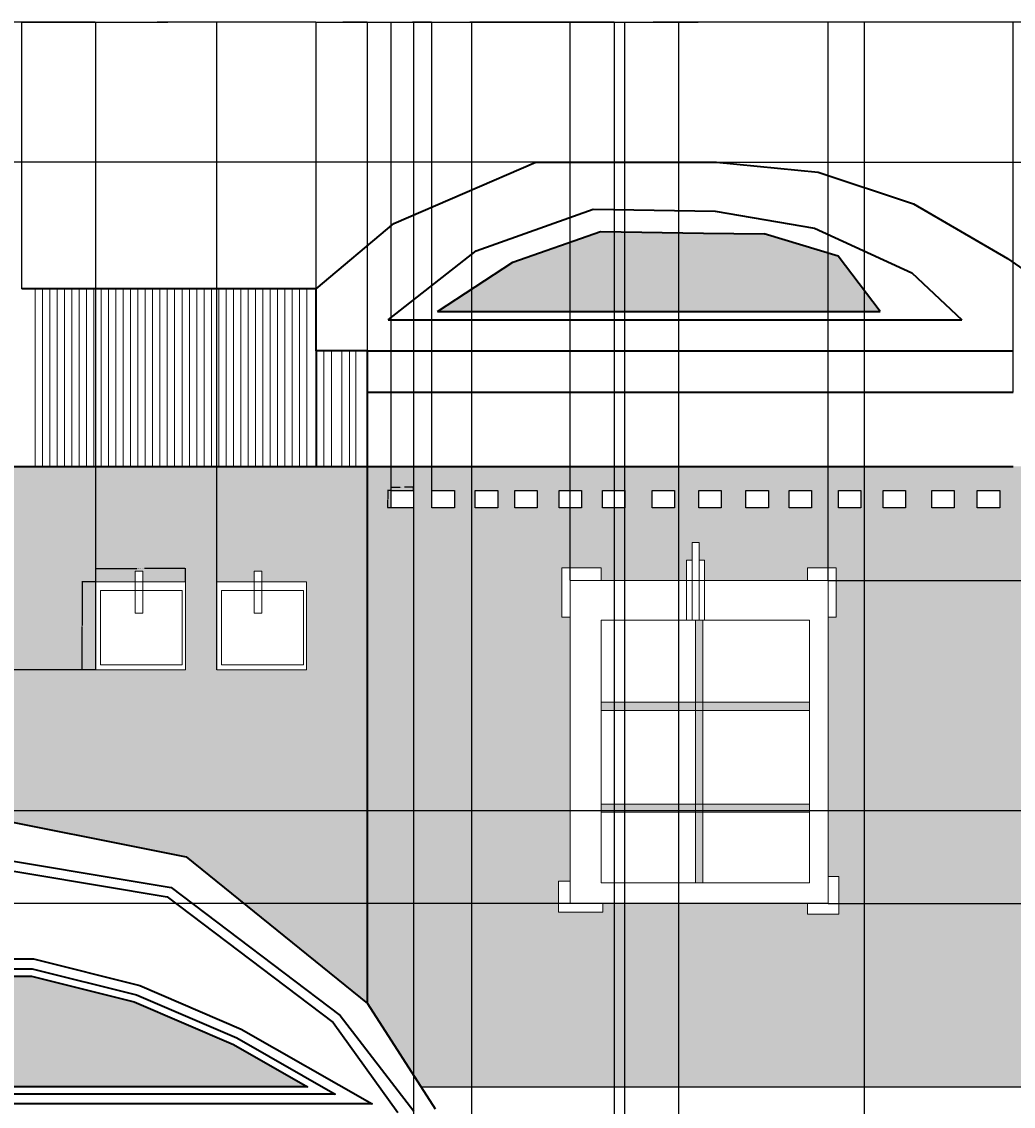
# Model space of a CAD drawing. Units: inches. Extents: x -46 to 1209, y 110 to 778.
# Tile 3 of 5: x 247 to 652, y 334 to 778. Entities that reach past the tile are written whole.
import ezdxf

# ---------------------------------------------------------------- set-up
doc = ezdxf.new("R2010")
doc.units = ezdxf.units.IN
doc.header["$MEASUREMENT"] = 0
for name, color, linetype, lineweight in [('A-ANNO-DIMS', 2, 'Continuous', 18), ('A-GLAZ', 4, 'Continuous', 20), ('A-GLAZ-PATT', 9, 'Continuous', 13), ('A-ROOF', 7, 'Continuous', 35), ('A-ROOF-PATT', 8, 'Continuous', 13), ('A-WALL', 7, 'Continuous', 35), ('A-WALL-PATT', 252, 'Continuous', 13), ('A-WALL-TRIM', 42, 'Continuous', 25)]:
    doc.layers.add(name, color=color, linetype=linetype, lineweight=lineweight)
doc.styles.get("Standard").update_dxf_attribs({"font": 'arial.ttf'})
doc.dimstyles.get("Standard").update_dxf_attribs({"dimtxt": 0.18, "dimasz": 0.18, "dimexe": 0.18, "dimexo": 0.0625, "dimgap": 0.09, "dimtad": 0, "dimtih": 1, "dimtoh": 1, "dimdec": 4, "dimzin": 0, "dimdsep": 46, "dimtxsty": 'Standard', "dimcen": 0.09, "dimadec": 0, "dimazin": 0, "dimtfac": 1, "dimtdec": 4, "dimtofl": 0, "dimtmove": 0, "dimatfit": 3, "dimfxl": 1, "dimtolj": 1, "dimtzin": 0, "dimarcsym": 0})

# ---------------------------------------------------------------- blocks, each defined once
blk = doc.blocks.new('WIN-SMALL-FRAME')
for points in [[(0, 35.97), (36.6, 35.97), (36.6, 0), (0, 0)], [(1.9, 32.4), (35.37, 32.4), (35.37, 2.05), (1.9, 2.05)]]:
    blk.add_lwpolyline(points, close=True)
blk = doc.blocks.new('DENTIL-FACADE')
blk.add_lwpolyline([(0, 7.16), (9.17, 7.16), (9.17, 0), (0, 0)], close=True)
blk = doc.blocks.new('*D12')
at = {"layer": 'A-ANNO-DIMS', "color": 0, "lineweight": -2, "transparency": 16777216}
for p, q in [((397.42, 586.03), (397.42, 587.53)), ((397.6, 587.35), (401.07, 587.35)), ((406.42, 587.35), (402.94, 587.35)), ((406.6, 586.03), (406.6, 587.53))]:
    blk.add_line(p, q, dxfattribs=at)
at = {"layer": 'A-ANNO-DIMS', "color": 0, "transparency": 16777216}
for points in [[(397.6, 587.38), (397.6, 587.32), (397.42, 587.35)], [(406.42, 587.38), (406.42, 587.32), (406.6, 587.35)]]:
    blk.add_solid(points, dxfattribs=at)
at = {"layer": 'Defpoints', "color": 0, "transparency": 16777216}
for p in [(397.42, 585.97), (406.6, 587.35), (406.6, 585.97)]:
    blk.add_point(p, dxfattribs=at)
at = {"layer": 'A-ANNO-DIMS', "color": 0, "transparency": 16777216, "insert": (402.01, 587.35), "char_height": 0.18, "attachment_point": 5}
blk.add_mtext('\\A1;DENTIL 9 TYP.', dxfattribs=at)
blk = doc.blocks.new('*D13')
at = {"layer": 'A-ANNO-DIMS', "color": 0, "lineweight": -2, "transparency": 16777216}
for p, q in [((397.36, 585.97), (395.87, 585.97)), ((396.05, 585.79), (396.05, 582.57)), ((396.05, 578.99), (396.05, 582.21)), ((397.36, 578.81), (395.87, 578.81))]:
    blk.add_line(p, q, dxfattribs=at)
at = {"layer": 'A-ANNO-DIMS', "color": 0, "transparency": 16777216}
for points in [[(396.02, 585.79), (396.08, 585.79), (396.05, 585.97)], [(396.02, 578.99), (396.08, 578.99), (396.05, 578.81)]]:
    blk.add_solid(points, dxfattribs=at)
at = {"layer": 'Defpoints', "color": 0, "transparency": 16777216}
for p in [(396.05, 585.97), (397.42, 585.97), (397.42, 578.81)]:
    blk.add_point(p, dxfattribs=at)
at = {"layer": 'A-ANNO-DIMS', "color": 0, "transparency": 16777216, "insert": (396.05, 582.39), "char_height": 0.18, "attachment_point": 5}
blk.add_mtext('\\A1;7 TYP.', dxfattribs=at)
blk = doc.blocks.new('*D20')
at = {"layer": 'A-ANNO-DIMS', "color": 0, "lineweight": -2, "transparency": 16777216}
for p, q in [((276.76, 548.66), (276.76, 554.27)), ((313.37, 548.66), (313.37, 554.27)), ((276.94, 554.09), (293.5, 554.09)), ((313.19, 554.09), (296.63, 554.09))]:
    blk.add_line(p, q, dxfattribs=at)
at = {"layer": 'A-ANNO-DIMS', "color": 0, "transparency": 16777216}
for points in [[(276.94, 554.12), (276.94, 554.06), (276.76, 554.09)], [(313.19, 554.12), (313.19, 554.06), (313.37, 554.09)]]:
    blk.add_solid(points, dxfattribs=at)
at = {"layer": 'Defpoints', "color": 0, "transparency": 16777216}
for p in [(313.37, 554.09), (276.76, 548.59), (313.37, 548.59)]:
    blk.add_point(p, dxfattribs=at)
at = {"layer": 'A-ANNO-DIMS', "color": 0, "transparency": 16777216, "insert": (295.07, 554.09), "char_height": 0.18, "attachment_point": 5}
blk.add_mtext('\\A1;SMALL WINDOW 37 TYP.', dxfattribs=at)
blk = doc.blocks.new('*D21')
at = {"layer": 'A-ANNO-DIMS', "color": 0, "lineweight": -2, "transparency": 16777216}
for p, q in [((276.7, 548.59), (271.09, 548.59)), ((271.27, 548.41), (271.27, 530.79)), ((271.27, 512.81), (271.27, 530.43)), ((276.7, 512.63), (271.09, 512.63))]:
    blk.add_line(p, q, dxfattribs=at)
at = {"layer": 'A-ANNO-DIMS', "color": 0, "transparency": 16777216}
for points in [[(271.24, 548.41), (271.3, 548.41), (271.27, 548.59)], [(271.24, 512.81), (271.3, 512.81), (271.27, 512.63)]]:
    blk.add_solid(points, dxfattribs=at)
at = {"layer": 'Defpoints', "color": 0, "transparency": 16777216}
for p in [(271.27, 548.59), (276.76, 548.59), (276.76, 512.63)]:
    blk.add_point(p, dxfattribs=at)
at = {"layer": 'A-ANNO-DIMS', "color": 0, "transparency": 16777216, "insert": (271.27, 530.61), "char_height": 0.18, "attachment_point": 5}
blk.add_mtext('\\A1;36 TYP.', dxfattribs=at)
blk = doc.blocks.new('*D29')
at = {"layer": 'A-ANNO-DIMS', "color": 0, "lineweight": -2, "transparency": 16777216}
for p, q in [((456.52, 720.07), (-45.5, 720.07)), ((-45.32, 719.89), (-45.32, 443.93)), ((-45.32, 167.62), (-45.32, 443.57)), ((15.16, 167.44), (-45.5, 167.44))]:
    blk.add_line(p, q, dxfattribs=at)
at = {"layer": 'A-ANNO-DIMS', "color": 0, "transparency": 16777216}
for points in [[(-45.35, 719.89), (-45.29, 719.89), (-45.32, 720.07)], [(-45.35, 167.62), (-45.29, 167.62), (-45.32, 167.44)]]:
    blk.add_solid(points, dxfattribs=at)
at = {"layer": 'Defpoints', "color": 0, "transparency": 16777216}
for p in [(-45.32, 720.07), (456.58, 720.07), (15.23, 167.44)]:
    blk.add_point(p, dxfattribs=at)
at = {"layer": 'A-ANNO-DIMS', "color": 0, "transparency": 16777216, "insert": (-45.32, 443.75), "char_height": 0.18, "attachment_point": 5}
blk.add_mtext('\\A1;552.6', dxfattribs=at)
blk = doc.blocks.new('*D46')
at = {"layer": 'A-ANNO-DIMS', "color": 0, "lineweight": -2, "transparency": 16777216}
for p, q in [((406.65, 322.05), (406.65, 777.55)), ((406.83, 777.37), (447.43, 777.37)), ((488.47, 777.37), (447.87, 777.37)), ((488.65, 273.58), (488.65, 777.55))]:
    blk.add_line(p, q, dxfattribs=at)
at = {"layer": 'A-ANNO-DIMS', "color": 0, "transparency": 16777216}
for points in [[(406.83, 777.4), (406.83, 777.34), (406.65, 777.37)], [(488.47, 777.4), (488.47, 777.34), (488.65, 777.37)]]:
    blk.add_solid(points, dxfattribs=at)
at = {"layer": 'Defpoints', "color": 0, "transparency": 16777216}
for p in [(488.65, 777.37), (406.65, 321.99), (488.65, 273.51)]:
    blk.add_point(p, dxfattribs=at)
at = {"layer": 'A-ANNO-DIMS', "color": 0, "transparency": 16777216, "insert": (447.65, 777.37), "char_height": 0.18, "attachment_point": 5}
blk.add_mtext('\\A1;82', dxfattribs=at)
blk = doc.blocks.new('*D50')
at = {"layer": 'A-ANNO-DIMS', "color": 0, "lineweight": -2, "transparency": 16777216}
for p, q in [((430.32, 322.05), (430.32, 777.55)), ((430.5, 777.37), (510.13, 777.37)), ((590.53, 777.37), (510.9, 777.37)), ((590.71, 322.05), (590.71, 777.55))]:
    blk.add_line(p, q, dxfattribs=at)
at = {"layer": 'A-ANNO-DIMS', "color": 0, "transparency": 16777216}
for points in [[(430.5, 777.4), (430.5, 777.34), (430.32, 777.37)], [(590.53, 777.4), (590.53, 777.34), (590.71, 777.37)]]:
    blk.add_solid(points, dxfattribs=at)
at = {"layer": 'Defpoints', "color": 0, "transparency": 16777216}
for p in [(590.71, 777.37), (430.32, 321.99), (590.71, 321.99)]:
    blk.add_point(p, dxfattribs=at)
at = {"layer": 'A-ANNO-DIMS', "color": 0, "transparency": 16777216, "insert": (510.52, 777.37), "char_height": 0.18, "attachment_point": 5}
blk.add_mtext('\\A1;160.4', dxfattribs=at)
blk = doc.blocks.new('*D51')
at = {"layer": 'A-ANNO-DIMS', "color": 0, "lineweight": -2, "transparency": 16777216}
for p, q in [((492.93, 261.94), (492.93, 777.55)), ((493.11, 777.37), (503.47, 777.37)), ((514.76, 777.37), (504.4, 777.37)), ((514.94, 261.94), (514.94, 777.55))]:
    blk.add_line(p, q, dxfattribs=at)
at = {"layer": 'A-ANNO-DIMS', "color": 0, "transparency": 16777216}
for points in [[(493.11, 777.4), (493.11, 777.34), (492.93, 777.37)], [(514.76, 777.4), (514.76, 777.34), (514.94, 777.37)]]:
    blk.add_solid(points, dxfattribs=at)
at = {"layer": 'Defpoints', "color": 0, "transparency": 16777216}
for p in [(514.94, 777.37), (492.93, 261.87), (514.94, 261.87)]:
    blk.add_point(p, dxfattribs=at)
at = {"layer": 'A-ANNO-DIMS', "color": 0, "transparency": 16777216, "insert": (503.94, 777.37), "char_height": 0.18, "attachment_point": 5}
blk.add_mtext('\\A1;22.003', dxfattribs=at)
blk = doc.blocks.new('*D59')
at = {"layer": 'A-ANNO-DIMS', "color": 0, "lineweight": -2, "transparency": 16777216}
for p, q in [((530.31, 720.07), (1209.28, 720.07)), ((1209.1, 719.89), (1209.1, 694.37)), ((1209.1, 668.48), (1209.1, 694)), ((1091.9, 668.3), (1209.28, 668.3))]:
    blk.add_line(p, q, dxfattribs=at)
at = {"layer": 'A-ANNO-DIMS', "color": 0, "transparency": 16777216}
for points in [[(1209.07, 719.89), (1209.13, 719.89), (1209.1, 720.07)], [(1209.07, 668.48), (1209.13, 668.48), (1209.1, 668.3)]]:
    blk.add_solid(points, dxfattribs=at)
at = {"layer": 'Defpoints', "color": 0, "transparency": 16777216}
for p in [(530.25, 720.07), (1209.1, 720.07), (1091.84, 668.3)]:
    blk.add_point(p, dxfattribs=at)
at = {"layer": 'A-ANNO-DIMS', "color": 0, "transparency": 16777216, "insert": (1209.1, 694.19), "char_height": 0.18, "attachment_point": 5}
blk.add_mtext('\\A1;51.77', dxfattribs=at)
blk = doc.blocks.new('*D61')
at = {"layer": 'A-ANNO-DIMS', "color": 0, "lineweight": -2, "transparency": 16777216}
for p, q in [((179.04, 595.79), (-45.5, 595.79)), ((-45.32, 595.61), (-45.32, 554.39)), ((-45.32, 512.81), (-45.32, 554.03)), ((276.7, 512.63), (-45.5, 512.63))]:
    blk.add_line(p, q, dxfattribs=at)
at = {"layer": 'A-ANNO-DIMS', "color": 0, "transparency": 16777216}
for points in [[(-45.35, 595.61), (-45.29, 595.61), (-45.32, 595.79)], [(-45.35, 512.81), (-45.29, 512.81), (-45.32, 512.63)]]:
    blk.add_solid(points, dxfattribs=at)
at = {"layer": 'Defpoints', "color": 0, "transparency": 16777216}
for p in [(179.1, 595.79), (-45.32, 512.63), (276.76, 512.63)]:
    blk.add_point(p, dxfattribs=at)
at = {"layer": 'A-ANNO-DIMS', "color": 0, "transparency": 16777216, "insert": (-45.32, 554.21), "char_height": 0.18, "attachment_point": 5}
blk.add_mtext('\\A1;83.16', dxfattribs=at)
blk = doc.blocks.new('*D62')
at = {"layer": 'A-ANNO-DIMS', "color": 0, "lineweight": -2, "transparency": 16777216}
for p, q in [((179.1, 595.85), (179.1, 777.55)), ((179.28, 777.37), (227.54, 777.37)), ((276.58, 777.37), (228.33, 777.37)), ((276.76, 512.69), (276.76, 777.55))]:
    blk.add_line(p, q, dxfattribs=at)
at = {"layer": 'A-ANNO-DIMS', "color": 0, "transparency": 16777216}
for points in [[(179.28, 777.4), (179.28, 777.34), (179.1, 777.37)], [(276.58, 777.4), (276.58, 777.34), (276.76, 777.37)]]:
    blk.add_solid(points, dxfattribs=at)
at = {"layer": 'Defpoints', "color": 0, "transparency": 16777216}
for p in [(276.76, 777.37), (179.1, 595.79), (276.76, 512.63)]:
    blk.add_point(p, dxfattribs=at)
at = {"layer": 'A-ANNO-DIMS', "color": 0, "transparency": 16777216, "insert": (227.93, 777.37), "char_height": 0.18, "attachment_point": 5}
blk.add_mtext('\\A1;97.66', dxfattribs=at)
blk = doc.blocks.new('*D63')
at = {"layer": 'A-ANNO-DIMS', "color": 0, "lineweight": -2, "transparency": 16777216}
for p, q in [((276.76, 512.69), (276.76, 777.55)), ((276.94, 777.37), (301.19, 777.37)), ((326.09, 777.37), (301.84, 777.37)), ((326.27, 512.69), (326.27, 777.55))]:
    blk.add_line(p, q, dxfattribs=at)
at = {"layer": 'A-ANNO-DIMS', "color": 0, "transparency": 16777216}
for points in [[(276.94, 777.4), (276.94, 777.34), (276.76, 777.37)], [(326.09, 777.4), (326.09, 777.34), (326.27, 777.37)]]:
    blk.add_solid(points, dxfattribs=at)
at = {"layer": 'Defpoints', "color": 0, "transparency": 16777216}
for p in [(326.27, 777.37), (276.76, 512.63), (326.27, 512.63)]:
    blk.add_point(p, dxfattribs=at)
at = {"layer": 'A-ANNO-DIMS', "color": 0, "transparency": 16777216, "insert": (301.52, 777.37), "char_height": 0.18, "attachment_point": 5}
blk.add_mtext('\\A1;49.5', dxfattribs=at)
blk = doc.blocks.new('*D64')
at = {"layer": 'A-ANNO-DIMS', "color": 0, "lineweight": -2, "transparency": 16777216}
for p, q in [((387.83, 595.85), (387.83, 777.55)), ((388.01, 777.37), (428.78, 777.37)), ((470.33, 777.37), (429.56, 777.37)), ((470.51, 549.26), (470.51, 777.55))]:
    blk.add_line(p, q, dxfattribs=at)
at = {"layer": 'A-ANNO-DIMS', "color": 0, "transparency": 16777216}
for points in [[(388.01, 777.4), (388.01, 777.34), (387.83, 777.37)], [(470.33, 777.4), (470.33, 777.34), (470.51, 777.37)]]:
    blk.add_solid(points, dxfattribs=at)
at = {"layer": 'Defpoints', "color": 0, "transparency": 16777216}
for p in [(470.51, 777.37), (387.83, 595.79), (470.51, 549.2)]:
    blk.add_point(p, dxfattribs=at)
at = {"layer": 'A-ANNO-DIMS', "color": 0, "transparency": 16777216, "insert": (429.17, 777.37), "char_height": 0.18, "attachment_point": 5}
blk.add_mtext('\\A1;82.68', dxfattribs=at)
blk = doc.blocks.new('*D65')
at = {"layer": 'A-ANNO-DIMS', "color": 0, "lineweight": -2, "transparency": 16777216}
for p, q in [((470.51, 549.26), (470.51, 777.55)), ((470.69, 777.37), (522.76, 777.37)), ((575.74, 777.37), (523.67, 777.37)), ((575.92, 549.26), (575.92, 777.55))]:
    blk.add_line(p, q, dxfattribs=at)
at = {"layer": 'A-ANNO-DIMS', "color": 0, "transparency": 16777216}
for points in [[(470.69, 777.4), (470.69, 777.34), (470.51, 777.37)], [(575.74, 777.4), (575.74, 777.34), (575.92, 777.37)]]:
    blk.add_solid(points, dxfattribs=at)
at = {"layer": 'Defpoints', "color": 0, "transparency": 16777216}
for p in [(575.92, 777.37), (470.51, 549.2), (575.92, 549.2)]:
    blk.add_point(p, dxfattribs=at)
at = {"layer": 'A-ANNO-DIMS', "color": 0, "transparency": 16777216, "insert": (523.22, 777.37), "char_height": 0.18, "attachment_point": 5}
blk.add_mtext('\\A1;105.42', dxfattribs=at)
blk = doc.blocks.new('*D66')
at = {"layer": 'A-ANNO-DIMS', "color": 0, "lineweight": -2, "transparency": 16777216}
for p, q in [((575.99, 549.2), (1209.28, 549.2)), ((1209.1, 549.02), (1209.1, 483.35)), ((1209.1, 417.31), (1209.1, 482.99)), ((575.99, 417.13), (1209.28, 417.13))]:
    blk.add_line(p, q, dxfattribs=at)
at = {"layer": 'A-ANNO-DIMS', "color": 0, "transparency": 16777216}
for points in [[(1209.07, 549.02), (1209.13, 549.02), (1209.1, 549.2)], [(1209.07, 417.31), (1209.13, 417.31), (1209.1, 417.13)]]:
    blk.add_solid(points, dxfattribs=at)
at = {"layer": 'Defpoints', "color": 0, "transparency": 16777216}
for p in [(575.92, 549.2), (1209.1, 549.2), (575.92, 417.13)]:
    blk.add_point(p, dxfattribs=at)
at = {"layer": 'A-ANNO-DIMS', "color": 0, "transparency": 16777216, "insert": (1209.1, 483.17), "char_height": 0.18, "attachment_point": 5}
blk.add_mtext('\\A1;132.07', dxfattribs=at)
blk = doc.blocks.new('*D67')
at = {"layer": 'A-ANNO-DIMS', "color": 0, "lineweight": -2, "transparency": 16777216}
for p, q in [((683.9, 455.08), (-45.5, 455.08)), ((-45.32, 454.9), (-45.32, 436.29)), ((-45.32, 417.31), (-45.32, 435.93)), ((575.86, 417.13), (-45.5, 417.13))]:
    blk.add_line(p, q, dxfattribs=at)
at = {"layer": 'A-ANNO-DIMS', "color": 0, "transparency": 16777216}
for points in [[(-45.35, 454.9), (-45.29, 454.9), (-45.32, 455.08)], [(-45.35, 417.31), (-45.29, 417.31), (-45.32, 417.13)]]:
    blk.add_solid(points, dxfattribs=at)
at = {"layer": 'Defpoints', "color": 0, "transparency": 16777216}
for p in [(-45.32, 455.08), (683.96, 455.08), (575.92, 417.13)]:
    blk.add_point(p, dxfattribs=at)
at = {"layer": 'A-ANNO-DIMS', "color": 0, "transparency": 16777216, "insert": (-45.32, 436.11), "char_height": 0.18, "attachment_point": 5}
blk.add_mtext('\\A1;37.95', dxfattribs=at)
blk = doc.blocks.new('*D74')
at = {"layer": 'A-ANNO-DIMS', "color": 0, "lineweight": -2, "transparency": 16777216}
for p, q in [((397.42, 578.88), (397.42, 777.55)), ((397.6, 777.37), (405.37, 777.37)), ((413.91, 777.37), (406.14, 777.37)), ((414.09, 578.88), (414.09, 777.55))]:
    blk.add_line(p, q, dxfattribs=at)
at = {"layer": 'A-ANNO-DIMS', "color": 0, "transparency": 16777216}
for points in [[(397.6, 777.4), (397.6, 777.34), (397.42, 777.37)], [(413.91, 777.4), (413.91, 777.34), (414.09, 777.37)]]:
    blk.add_solid(points, dxfattribs=at)
at = {"layer": 'Defpoints', "color": 0, "transparency": 16777216}
for p in [(414.09, 777.37), (397.42, 578.81), (414.09, 578.81)]:
    blk.add_point(p, dxfattribs=at)
at = {"layer": 'A-ANNO-DIMS', "color": 0, "transparency": 16777216, "insert": (405.76, 777.37), "char_height": 0.18, "attachment_point": 5}
blk.add_mtext('\\A1;16.67', dxfattribs=at)
blk = doc.blocks.new('*D75')
at = {"layer": 'A-ANNO-DIMS', "color": 0, "lineweight": -2, "transparency": 16777216}
for p, q in [((387.83, 626.19), (387.83, 777.55)), ((388.01, 777.37), (519.29, 777.37)), ((651.36, 777.37), (520.08, 777.37)), ((651.54, 626.19), (651.54, 777.55))]:
    blk.add_line(p, q, dxfattribs=at)
at = {"layer": 'A-ANNO-DIMS', "color": 0, "transparency": 16777216}
for points in [[(388.01, 777.4), (388.01, 777.34), (387.83, 777.37)], [(651.36, 777.4), (651.36, 777.34), (651.54, 777.37)]]:
    blk.add_solid(points, dxfattribs=at)
at = {"layer": 'Defpoints', "color": 0, "transparency": 16777216}
for p in [(651.54, 777.37), (387.83, 626.13), (651.54, 626.13)]:
    blk.add_point(p, dxfattribs=at)
at = {"layer": 'A-ANNO-DIMS', "color": 0, "transparency": 16777216, "insert": (519.68, 777.37), "char_height": 0.18, "attachment_point": 5}
blk.add_mtext('\\A1;263.7', dxfattribs=at)
blk = doc.blocks.new('*D76')
at = {"layer": 'A-ANNO-DIMS', "color": 0, "lineweight": -2, "transparency": 16777216}
for p, q in [((366.79, 643.05), (366.79, 777.55)), ((366.97, 777.37), (376.92, 777.37)), ((387.65, 777.37), (377.71, 777.37)), ((387.83, 626.19), (387.83, 777.55))]:
    blk.add_line(p, q, dxfattribs=at)
at = {"layer": 'A-ANNO-DIMS', "color": 0, "transparency": 16777216}
for points in [[(366.97, 777.4), (366.97, 777.34), (366.79, 777.37)], [(387.65, 777.4), (387.65, 777.34), (387.83, 777.37)]]:
    blk.add_solid(points, dxfattribs=at)
at = {"layer": 'Defpoints', "color": 0, "transparency": 16777216}
for p in [(387.83, 777.37), (366.79, 642.99), (387.83, 626.13)]:
    blk.add_point(p, dxfattribs=at)
at = {"layer": 'A-ANNO-DIMS', "color": 0, "transparency": 16777216, "insert": (377.31, 777.37), "char_height": 0.18, "attachment_point": 5}
blk.add_mtext('\\A1;21.04', dxfattribs=at)
blk = doc.blocks.new('*D77')
at = {"layer": 'A-ANNO-DIMS', "color": 0, "lineweight": -2, "transparency": 16777216}
for p, q in [((246.53, 668.36), (246.53, 777.55)), ((246.71, 777.37), (306.21, 777.37)), ((366.61, 777.37), (307.12, 777.37)), ((366.79, 668.36), (366.79, 777.55))]:
    blk.add_line(p, q, dxfattribs=at)
at = {"layer": 'A-ANNO-DIMS', "color": 0, "transparency": 16777216}
for points in [[(246.71, 777.4), (246.71, 777.34), (246.53, 777.37)], [(366.61, 777.4), (366.61, 777.34), (366.79, 777.37)]]:
    blk.add_solid(points, dxfattribs=at)
at = {"layer": 'Defpoints', "color": 0, "transparency": 16777216}
for p in [(366.79, 777.37), (246.53, 668.3), (366.79, 668.3)]:
    blk.add_point(p, dxfattribs=at)
at = {"layer": 'A-ANNO-DIMS', "color": 0, "transparency": 16777216, "insert": (306.66, 777.37), "char_height": 0.18, "attachment_point": 5}
blk.add_mtext('\\A1;120.26', dxfattribs=at)
blk = doc.blocks.new('*D78')
at = {"layer": 'A-ANNO-DIMS', "color": 0, "lineweight": -2, "transparency": 16777216}
for p, q in [((366.79, 643.05), (366.79, 777.55)), ((366.97, 777.37), (517.24, 777.37)), ((668.29, 777.37), (518.02, 777.37)), ((668.47, 643.05), (668.47, 777.55))]:
    blk.add_line(p, q, dxfattribs=at)
at = {"layer": 'A-ANNO-DIMS', "color": 0, "transparency": 16777216}
for points in [[(366.97, 777.4), (366.97, 777.34), (366.79, 777.37)], [(668.29, 777.4), (668.29, 777.34), (668.47, 777.37)]]:
    blk.add_solid(points, dxfattribs=at)
at = {"layer": 'Defpoints', "color": 0, "transparency": 16777216}
for p in [(668.47, 777.37), (366.79, 642.99), (668.47, 642.99)]:
    blk.add_point(p, dxfattribs=at)
at = {"layer": 'A-ANNO-DIMS', "color": 0, "transparency": 16777216, "insert": (517.63, 777.37), "char_height": 0.18, "attachment_point": 5}
blk.add_mtext('\\A1;301.7', dxfattribs=at)

msp = doc.modelspace()

# ---------------------------------------------------------------- hatches: boundary and pattern name
at = {"layer": 'A-GLAZ-PATT'}
h = msp.add_hatch(color=256, dxfattribs=at)
h.dxf.hatch_style = 1
h.paths.add_polyline_path([(524.7711, 532.926), (523.2165, 532.926), (521.7711, 532.926), (521.7711, 499.4601), (524.7711, 499.4601)])
h.paths.add_polyline_path([(524.7711, 499.4601), (521.7711, 499.4601), (521.7711, 496.0287), (524.7711, 496.0287)])
h.paths.add_polyline_path([(568.2834, 499.4601), (524.7711, 499.4601), (524.7711, 496.0287), (568.2834, 496.0287)])
h.paths.add_polyline_path([(521.7711, 499.4601), (483.2375, 499.4601), (483.2375, 496.0287), (521.7711, 496.0287)])
h.paths.add_polyline_path([(524.7711, 496.0287), (521.7711, 496.0287), (521.7711, 425.5857), (524.7711, 425.5857)])
h.paths.add_polyline_path([(568.2834, 457.8123), (524.7711, 457.8123), (524.7711, 454.4649), (568.2834, 454.4649)])
h.paths.add_polyline_path([(521.7711, 457.8123), (483.2375, 457.8123), (483.2375, 454.4649), (521.7711, 454.4649)])
h.paths.add_polyline_path([(741.5274, 266.4582), (707.3294, 266.4582), (707.3294, 263.369), (741.5274, 263.369)])
h.paths.add_polyline_path([(741.5274, 236.0814), (707.3294, 236.0814), (707.3294, 232.9922), (741.5274, 232.9922)])
h.paths.add_polyline_path([(898.2871, 266.4582), (864.0892, 266.4582), (864.0892, 263.369), (898.2871, 263.369)])
h.paths.add_polyline_path([(898.2871, 236.0814), (864.0892, 236.0814), (864.0892, 232.9922), (898.2871, 232.9922)])
h.paths.add_polyline_path([(1052.6765, 266.4582), (1018.4786, 266.4582), (1018.4786, 263.369), (1052.6765, 263.369)])
h.paths.add_polyline_path([(1052.6765, 236.0814), (1018.4786, 236.0814), (1018.4786, 232.9922), (1052.6765, 232.9922)])
at = {"layer": 'A-ROOF-PATT'}
h = msp.add_hatch(dxfattribs=at)
h.set_pattern_fill('ANSI31', color=256, scale=24, angle=45, style=0)
h.paths.add_polyline_path([(249.0671, 595.7911), (363.0671, 595.7911), (363.0671, 668.3019), (249.0671, 668.3019)])
at = {"layer": 'A-WALL-PATT'}
h = msp.add_hatch(dxfattribs=at)
h.set_pattern_fill('AR-CONC', color=256, scale=3)
h.paths.add_polyline_path([(387.8322, 595.7911), (179.1007, 595.7911), (179.1007, 451.7911), (179.1007, 439.7911), (220.892, 454.7186), (313.6366, 436.1845), (387.8322, 376.346)])
h.paths.add_polyline_path([(276.7646, 548.5945), (292.8821, 548.5945), (292.8821, 553.0308), (295.9402, 553.0308), (295.9402, 548.5945), (313.3682, 548.5945), (313.3682, 512.6263), (276.7646, 512.6263)], flags=16)
h.paths.add_polyline_path([(278.6627, 545.0233), (312.1316, 545.0233), (312.1316, 514.6792), (278.6627, 514.6792)], flags=0)
h.paths.add_polyline_path([(326.2691, 548.5945), (341.5129, 548.5945), (341.5129, 553.0308), (344.571, 553.0308), (344.571, 548.5945), (362.8728, 548.5945), (362.8728, 512.6263), (326.2691, 512.6263)], flags=16)
h.paths.add_polyline_path([(328.1673, 545.0233), (361.6362, 545.0233), (361.6362, 514.6792), (328.1673, 514.6792)], flags=0)
h.paths.add_polyline_path([(651.5361, 595.7911), (415.401, 595.7911), (387.8322, 595.7911), (387.8322, 376.346), (409.6414, 342.2631), (651.5361, 342.2631)])
h.paths.add_polyline_path([(470.5081, 534.2042), (467.0793, 534.2042), (467.0793, 554.4029), (483.2058, 554.4029), (483.2058, 549.2024), (518.0634, 549.2024), (518.0634, 557.4852), (520.3257, 557.4852), (520.3257, 564.6435), (523.2165, 564.6435), (523.2165, 557.4852), (525.4788, 557.4852), (525.4788, 549.2024), (567.4184, 549.2024), (567.4184, 554.4029), (579.1691, 554.4029), (579.1691, 534.2042), (575.9249, 534.2042), (575.9249, 428.1662), (580.259, 428.1662), (580.259, 412.8567), (567.4184, 412.8567), (567.4184, 417.1318), (483.8186, 417.1318), (483.8186, 413.5449), (465.7589, 413.5449), (465.7589, 426.3336), (470.5081, 426.3336)], flags=16)
h.paths.add_polyline_path([(483.2375, 532.926), (568.2834, 532.926), (568.2834, 425.5857), (483.2375, 425.5857)], flags=0)
h.paths.add_polyline_path([(431.7717, 578.8147), (431.7717, 585.9699), (440.9467, 585.9699), (440.9467, 578.8147)], flags=16)
h.paths.add_polyline_path([(423.2681, 578.8147), (414.0931, 578.8147), (414.0931, 585.9699), (423.2681, 585.9699)], flags=16)
h.paths.add_polyline_path([(447.8839, 578.8147), (447.8839, 585.9699), (457.0589, 585.9699), (457.0589, 578.8147)], flags=16)
h.paths.add_polyline_path([(406.5964, 578.8147), (397.4214, 578.8147), (397.4214, 585.9699), (406.5964, 585.9699)], flags=16)
h.paths.add_polyline_path([(466.0101, 578.8147), (466.0101, 585.9699), (475.1851, 585.9699), (475.1851, 578.8147)], flags=16)
h.paths.add_polyline_path([(483.6888, 578.8147), (483.6888, 585.9699), (492.8638, 585.9699), (492.8638, 578.8147)], flags=16)
h.paths.add_polyline_path([(504.0528, 578.8147), (504.0528, 585.9699), (513.2278, 585.9699), (513.2278, 578.8147)], flags=16)
h.paths.add_polyline_path([(523.0742, 578.8147), (523.0742, 585.9699), (532.2492, 585.9699), (532.2492, 578.8147)], flags=16)
h.paths.add_polyline_path([(542.3193, 578.8147), (542.3193, 585.9699), (551.4943, 585.9699), (551.4943, 578.8147)], flags=16)
h.paths.add_polyline_path([(559.998, 578.8147), (559.998, 585.9699), (569.1729, 585.9699), (569.1729, 578.8147)], flags=16)
h.paths.add_polyline_path([(580.1382, 578.8147), (580.1382, 585.9699), (589.3132, 585.9699), (589.3132, 578.8147)], flags=16)
h.paths.add_polyline_path([(598.3313, 578.8147), (598.3313, 585.9699), (607.5063, 585.9699), (607.5063, 578.8147)], flags=16)
h.paths.add_polyline_path([(618.2477, 578.8147), (618.2477, 585.9699), (627.4227, 585.9699), (627.4227, 578.8147)], flags=16)
h.paths.add_polyline_path([(636.8215, 578.8147), (636.8215, 585.9699), (645.9965, 585.9699), (645.9965, 578.8147)], flags=16)
h.paths.add_polyline_path([(1151.8016, 595.7911), (651.5361, 595.7911), (651.5361, 342.2631), (939.9139, 342.2631), (1151.8016, 342.2631)])
h.paths.add_polyline_path([(683.9631, 455.0835), (683.9631, 537.4823), (720.8864, 537.4823), (720.8864, 547.6453), (727.8922, 547.6453), (727.8922, 537.4823), (767.8177, 537.4823), (767.8177, 455.0835)], flags=16)
h.paths.add_polyline_path([(688.3115, 459.7865), (688.3115, 529.3012), (764.9847, 529.3012), (764.9847, 459.7865)], flags=0)
h.paths.add_polyline_path([(840.5045, 455.0835), (840.5045, 537.4823), (877.4279, 537.4823), (877.4279, 547.6453), (884.4336, 547.6453), (884.4336, 537.4823), (924.3592, 537.4823), (924.3592, 455.0835)], flags=16)
h.paths.add_polyline_path([(844.853, 459.7865), (844.853, 529.3012), (921.5262, 529.3012), (921.5262, 459.7865)], flags=0)
h.paths.add_polyline_path([(994.2223, 455.0835), (994.2223, 537.4823), (1031.1457, 537.4823), (1031.1457, 547.6453), (1038.1514, 547.6453), (1038.1514, 537.4823), (1078.077, 537.4823), (1078.077, 455.0835)], flags=16)
h.paths.add_polyline_path([(998.5708, 459.7865), (998.5708, 529.3012), (1075.244, 529.3012), (1075.244, 459.7865)], flags=0)
h.paths.add_polyline_path([(1151.8016, 321.9907), (941.4829, 321.9907), (632.1261, 321.9907), (632.1261, 313.1625), (629.6322, 313.1625), (629.6322, 281.6236), (635.9059, 281.6236), (635.9059, 276.2471), (629.6322, 276.2471), (629.6322, 185.3878), (632.1261, 185.3878), (632.1261, 177.7316), (1151.8016, 177.7316)])
h.paths.add_polyline_path([(704.3294, 282.1806), (702.3037, 282.1806), (702.3037, 292.8947), (707.3294, 292.8947), (707.3294, 290.4743), (740.8704, 290.4743), (740.8704, 292.7856), (747.2108, 292.7856), (747.2108, 281.5404), (744.5274, 281.5404), (744.5274, 216.7007), (746.4513, 216.7007), (746.4513, 208.2103), (741.5274, 208.2103), (741.5274, 210.4615), (707.3294, 210.4615), (707.3294, 208.0997), (702.1613, 208.0997), (702.1613, 216.7007), (704.3294, 216.7007)], flags=16)
h.paths.add_polyline_path([(707.3294, 287.4743), (741.5274, 287.4743), (741.5274, 213.4615), (707.3294, 213.4615)], flags=0)
h.paths.add_polyline_path([(859.0635, 282.1806), (859.0635, 292.8947), (864.0892, 292.8947), (864.0892, 290.4743), (897.6301, 290.4743), (897.6301, 292.7856), (903.9705, 292.7856), (903.9705, 281.5404), (901.2871, 281.5404), (901.2871, 216.7007), (903.2111, 216.7007), (903.2111, 208.2103), (898.2871, 208.2103), (898.2871, 210.4615), (864.0892, 210.4615), (864.0892, 208.0997), (858.9211, 208.0997), (858.9211, 216.7007), (861.0892, 216.7007), (861.0892, 282.1806)], flags=16)
h.paths.add_polyline_path([(864.0892, 287.4743), (898.2871, 287.4743), (898.2871, 213.4615), (864.0892, 213.4615)], flags=0)
h.paths.add_polyline_path([(1013.4529, 282.1806), (1013.4529, 292.8947), (1018.4786, 292.8947), (1018.4786, 290.4743), (1052.0195, 290.4743), (1052.0195, 292.7856), (1058.3599, 292.7856), (1058.3599, 281.5404), (1055.6765, 281.5404), (1055.6765, 216.7007), (1057.6005, 216.7007), (1057.6005, 208.2103), (1052.6765, 208.2103), (1052.6765, 210.4615), (1018.4786, 210.4615), (1018.4786, 208.0997), (1013.3105, 208.0997), (1013.3105, 216.7007), (1015.4786, 216.7007), (1015.4786, 282.1806)], flags=16)
h.paths.add_polyline_path([(1018.4786, 287.4743), (1052.6765, 287.4743), (1052.6765, 213.4615), (1018.4786, 213.4615)], flags=0)
h.paths.add_polyline_path([(431.9367, 276.2471), (423.7231, 276.2471), (423.7231, 281.6236), (431.9367, 281.6236), (431.9367, 313.1625), (430.3199, 313.1625), (430.3199, 321.9907), (406.6462, 321.9907), (406.6462, 321.7316), (405.6256, 177.7316), (430.3199, 177.7316), (430.3199, 185.3878), (431.9367, 185.3878)])
h.paths.add_polyline_path([(406.6462, 321.7316), (406.6462, 321.9907), (363.2774, 321.9907), (58.5947, 321.7316), (57.7764, 206.2827), (87.7834, 206.0701), (87.7834, 290.4607), (89.9075, 293.33), (149.9611, 311.663), (149.9611, 316.8909), (153.3383, 316.8909), (153.3383, 311.1504), (213.2336, 293.3362), (215.3783, 290.4607), (215.3783, 205.1657), (246.588, 204.9445), (246.588, 290.0127), (248.7121, 292.882), (308.2509, 311.0579), (308.2509, 316.0122), (311.6281, 316.0122), (311.6281, 310.8556), (372.0381, 292.8882), (374.1829, 290.0127), (374.1829, 204.0402), (405.8105, 203.8161)])
h.paths.add_polyline_path([(333, 359.5), (292.5, 377), (250.5, 387.5), (199, 387.5), (155, 377.5), (123.5, 364), (101.4287, 342.2631), (363.2774, 342.2631)])
h.paths.add_polyline_path([(579.9721, 681.6773), (549.8011, 690.7996), (524.9646, 691.17), (482.8908, 691.7975), (447.0968, 679.2482), (416.3264, 659.1694), (597.1807, 659.1694)])

# ---------------------------------------------------------------- linework, layer by layer
at = {"layer": 'A-GLAZ'}
for p, q in [((483.2058, 554.4029), (467.0793, 554.4029)), ((467.0793, 554.4029), (467.0793, 534.2042)), ((483.2058, 549.2024), (483.2058, 554.4029)), ((567.4184, 549.2024), (567.4184, 554.4029)), ((567.4184, 554.4029), (579.1691, 554.4029)), ((579.1691, 554.4029), (579.1691, 534.2042)), ((467.0793, 534.2042), (470.5081, 534.2042)), ((521.7711, 532.926), (521.7711, 425.5857)), ((524.7711, 532.926), (524.7711, 425.5857)), ((579.1691, 534.2042), (575.9249, 534.2042)), ((483.2375, 499.4601), (568.2834, 499.4601)), ((483.2375, 496.0287), (568.2834, 496.0287)), ((483.2375, 457.8123), (568.2834, 457.8123)), ((483.2375, 454.4649), (568.2834, 454.4649)), ((465.7589, 413.5449), (465.7589, 426.3336)), ((465.7589, 426.3336), (470.5081, 426.3336)), ((580.259, 428.1662), (575.9249, 428.1662)), ((580.259, 412.8567), (580.259, 428.1662)), ((483.8186, 417.1318), (483.8186, 413.5449)), ((567.4184, 417.1318), (567.4184, 412.8567)), ((483.8186, 413.5449), (465.7589, 413.5449)), ((567.4184, 412.8567), (580.259, 412.8567))]:
    msp.add_line(p, q, dxfattribs=at)
for points in [[(520.3257, 564.6435), (523.2165, 564.6435), (523.2165, 532.926), (520.3257, 532.926)], [(518.0634, 557.4852), (520.3257, 557.4852), (520.3257, 532.926), (518.0634, 532.926)], [(523.2165, 557.4852), (525.4788, 557.4852), (525.4788, 532.926), (523.2165, 532.926)], [(292.8821, 553.0308), (295.9402, 553.0308), (295.9402, 535.808), (292.8821, 535.808)], [(341.5129, 553.0308), (344.571, 553.0308), (344.571, 535.808), (341.5129, 535.808)], [(470.5081, 549.2024), (575.9249, 549.2024), (575.9249, 417.1318), (470.5081, 417.1318)], [(483.2375, 532.926), (568.2834, 532.926), (568.2834, 425.5857), (483.2375, 425.5857)]]:
    msp.add_lwpolyline(points, close=True, dxfattribs=at)
at = {"layer": 'A-ROOF'}
for p, q in [((530.2452, 720.0699), (571.8615, 716.0337)), ((571.8615, 716.0337), (610.7245, 703.0897)), ((610.7245, 703.0897), (649.1949, 680.732)), ((649.1949, 680.732), (668.4684, 667.3071)), ((366.7938, 668.3019), (246.5295, 668.3019)), ((366.7938, 642.9876), (366.7938, 668.3019)), ((416.3264, 659.1694), (597.1807, 659.1694)), ((396.2651, 655.7064), (630.5263, 655.7064)), ((387.8322, 642.9876), (366.7938, 642.9876)), ((366.7938, 642.9876), (366.7938, 595.7911)), ((387.8322, 626.1254), (387.8322, 642.9876)), ((387.8322, 642.9876), (646.6805, 642.9876)), ((646.6805, 642.9876), (651.5361, 642.9876)), ((387.8322, 595.7911), (387.8322, 626.1254)), ((387.8322, 626.1254), (651.5361, 626.1254))]:
    msp.add_line(p, q, dxfattribs=at)
for points in [[(366.7938, 668.3019), (398.5302, 695.1202), (456.5847, 720.0699), (530.2452, 720.0699)], [(396.2651, 655.7064), (432.1084, 683.8464), (479.8993, 700.9009), (529.8239, 700.0482), (570.3608, 693.2264), (610.0444, 674.8927), (630.5263, 655.7064)], [(416.3264, 659.1694), (447.0968, 679.2482), (482.8908, 691.7975), (524.9646, 691.17), (549.8011, 690.7996), (549.8011, 690.7996)], [(597.1807, 659.1694), (579.9721, 681.6773), (549.8011, 690.7996)], [(53.8945, 337.7316), (104.7154, 413.2214), (220.892, 454.7186), (313.6366, 436.1845), (387.8322, 376.346), (415.401, 333.2621)], [(56.9823, 332.8507), (113.0259, 401.4848), (221.8022, 437.979), (307.5529, 423.6986), (376.6298, 371.3374), (406.7029, 332.2401)], [(61.2975, 331.811), (115.3935, 398.06), (222.1289, 433.8695), (305.9227, 419.915), (373.7332, 368.5138), (400.1222, 331.7916)]]:
    msp.add_lwpolyline(points, dxfattribs=at)
for points in [[(84.345, 335.2631), (119.5289, 369.9139), (152.8278, 384.1848), (198.2146, 394.5), (251.3617, 394.5), (294.7521, 383.6524), (336.1293, 365.7734), (389.722, 335.2631)], [(94.1071, 339.2631), (121.7981, 366.5345), (154.0691, 380.3649), (198.6634, 390.5), (250.8693, 390.5), (293.4652, 379.851), (334.3411, 362.1886), (374.6108, 339.2631)], [(101.4287, 342.2631), (123.5, 364), (155, 377.5), (199, 387.5), (250.5, 387.5), (292.5, 377), (333, 359.5), (363.2774, 342.2631)]]:
    msp.add_lwpolyline(points, close=True, dxfattribs=at)
at = {"layer": 'A-ROOF-PATT'}
for p, q in [((369.8774, 642.9876), (369.8774, 595.7911)), ((373.0413, 642.9876), (373.0413, 595.7911)), ((377.313, 642.9876), (377.313, 595.7911)), ((380.4237, 642.9876), (380.4237, 595.7911)), ((383.0603, 642.9876), (383.0603, 595.7911))]:
    msp.add_line(p, q, dxfattribs=at)
at = {"layer": 'A-WALL'}
for p, q in [((179.1007, 595.7911), (415.401, 595.7911)), ((387.8322, 376.346), (387.8322, 595.7911)), ((415.401, 595.7911), (651.5361, 595.7911))]:
    msp.add_line(p, q, dxfattribs=at)
at = {"layer": 'A-WALL-TRIM'}
msp.add_line((409.6414, 342.2631), (939.9139, 342.2631), dxfattribs=at)

# ---------------------------------------------------------------- block references
at = {"layer": 'A-GLAZ'}
for p in [(276.7646, 512.6263), (326.2691, 512.6263)]:
    msp.add_blockref('WIN-SMALL-FRAME', p, dxfattribs=at)
at = {"layer": 'A-WALL-TRIM'}
for p in [(397.4214, 578.8147), (414.0931, 578.8147), (431.7717, 578.8147), (447.8839, 578.8147), (466.0101, 578.8147), (483.6888, 578.8147), (504.0528, 578.8147), (523.0742, 578.8147), (542.3193, 578.8147), (559.998, 578.8147), (580.1382, 578.8147), (598.3313, 578.8147), (618.2477, 578.8147), (636.8215, 578.8147)]:
    msp.add_blockref('DENTIL-FACADE', p, dxfattribs=at)

# ---------------------------------------------------------------- dimensions: what is measured, and where the dimension line sits
at = {"layer": 'A-ANNO-DIMS'}
for base, p1, p2, override, picture, middle in [((276.7646, 777.3699), (179.1007, 595.7911), (276.7646, 512.6263), {"dimdec": 2, "dimlfac": 1, "dimrnd": 0, "dimzin": 0, "dimdsep": 46, "dimlunit": 2}, '*D62', (227.9326, 777.3699)), ((366.7938, 777.3699), (246.5295, 668.3019), (366.7938, 668.3019), {"dimdec": 2, "dimlfac": 1, "dimrnd": 0, "dimzin": 0, "dimdsep": 46, "dimlunit": 2}, '*D77', (306.6616, 777.3699)), ((326.2691, 777.3699), (276.7646, 512.6263), (326.2691, 512.6263), {"dimdec": 1, "dimlfac": 1, "dimrnd": 0, "dimzin": 0, "dimdsep": 46, "dimlunit": 2}, '*D63', (301.5169, 777.3699)), ((387.8322, 777.3699), (366.7938, 642.9876), (387.8322, 626.1254), {"dimdec": 2, "dimlfac": 1, "dimrnd": 0, "dimzin": 0, "dimdsep": 46, "dimlunit": 2}, '*D76', (377.313, 777.3699)), ((668.4684, 777.3699), (366.7938, 642.9876), (668.4684, 642.9876), {"dimdec": 1, "dimlfac": 1, "dimrnd": 0, "dimzin": 0, "dimdsep": 46, "dimlunit": 2}, '*D78', (517.6311, 777.3699)), ((470.5081, 777.3699), (387.8322, 595.7911), (470.5081, 549.2024), {"dimdec": 2, "dimlfac": 1, "dimrnd": 0, "dimzin": 0, "dimdsep": 46, "dimlunit": 2}, '*D64', (429.1701, 777.3699)), ((651.5361, 777.3699), (387.8322, 626.1254), (651.5361, 626.1254), {"dimdec": 1, "dimlfac": 1, "dimrnd": 0, "dimzin": 0, "dimdsep": 46, "dimlunit": 2}, '*D75', (519.6842, 777.3699)), ((414.0931, 777.3699), (397.4214, 578.8147), (414.0931, 578.8147), {"dimdec": 2, "dimlfac": 1, "dimrnd": 0, "dimzin": 0, "dimdsep": 46, "dimlunit": 2}, '*D74', (405.7572, 777.3699)), ((488.6503, 777.3699), (406.6462, 321.9907), (488.6503, 273.5127), {"dimdec": 0, "dimlfac": 1, "dimrnd": 0, "dimzin": 0, "dimdsep": 46, "dimlunit": 2}, '*D46', (447.6483, 777.3699)), ((590.712, 777.3699), (430.3199, 321.9907), (590.712, 321.9907), {"dimdec": 1, "dimlfac": 1, "dimrnd": 0, "dimzin": 0, "dimdsep": 46, "dimlunit": 2}, '*D50', (510.5159, 777.3699)), ((575.9249, 777.3699), (470.5081, 549.2024), (575.9249, 549.2024), {"dimdec": 2, "dimlfac": 1, "dimrnd": 0, "dimzin": 0, "dimdsep": 46, "dimlunit": 2}, '*D65', (523.2165, 777.3699)), ((514.9372, 777.3699), (492.9346, 261.8732), (514.9372, 261.8732), {"dimdec": 3, "dimlfac": 1, "dimrnd": 0, "dimzin": 0, "dimdsep": 46, "dimlunit": 2}, '*D51', (503.9359, 777.3699))]:
    dim = msp.add_linear_dim(base=base, p1=p1, p2=p2, dimstyle='Standard', override=override, dxfattribs=at)
    dim.commit()
    dim.dimension.update_dxf_attribs({"geometry": picture, "text_midpoint": middle})
for base, p1, p2, override, picture, middle in [((-45.3158, 720.0699), (15.2259, 167.435), (456.5847, 720.0699), {"dimdec": 1, "dimlfac": 1, "dimrnd": 0, "dimzin": 0, "dimdsep": 46, "dimlunit": 2}, '*D29', (-45.3158, 443.7524)), ((1209.1016, 720.0699), (1091.8408, 668.3019), (530.2452, 720.0699), {"dimdec": 2, "dimlfac": 1, "dimrnd": 0, "dimzin": 0, "dimdsep": 46, "dimlunit": 2}, '*D59', (1209.1016, 694.1859)), ((-45.3158, 512.6263), (179.1007, 595.7911), (276.7646, 512.6263), {"dimdec": 2, "dimlfac": 1, "dimrnd": 0, "dimzin": 0, "dimdsep": 46, "dimlunit": 2}, '*D61', (-45.3158, 554.2087)), ((1209.1016, 549.2024), (575.9249, 417.1318), (575.9249, 549.2024), {"dimdec": 2, "dimlfac": 1, "dimrnd": 0, "dimzin": 0, "dimdsep": 46, "dimlunit": 2}, '*D66', (1209.1016, 483.1671)), ((-45.3158, 455.0835), (575.9249, 417.1318), (683.9631, 455.0835), {"dimdec": 2, "dimlfac": 1, "dimrnd": 0, "dimzin": 0, "dimdsep": 46, "dimlunit": 2}, '*D67', (-45.3158, 436.1076))]:
    dim = msp.add_linear_dim(base=base, p1=p1, p2=p2, angle=90, dimstyle='Standard', override=override, dxfattribs=at)
    dim.commit()
    dim.dimension.update_dxf_attribs({"geometry": picture, "text_midpoint": middle})
for base, p1, p2, picture, middle in [((396.0452, 585.9699), (397.4214, 578.8147), (397.4214, 585.9699), '*D13', (396.0452, 582.3923)), ((271.274, 548.5945), (276.7646, 512.6263), (276.7646, 548.5945), '*D21', (271.274, 530.6104))]:
    dim = msp.add_linear_dim(base=base, p1=p1, p2=p2, angle=90, text='<> TYP.', dimstyle='Standard', override={"dimdec": 0, "dimlfac": 1, "dimrnd": 0, "dimzin": 0, "dimdsep": 46, "dimlunit": 2}, dxfattribs=at)
    dim.commit()
    dim.dimension.update_dxf_attribs({"geometry": picture, "text_midpoint": middle})
for base, p1, p2, text, picture, middle in [((406.5964, 587.3462), (397.4214, 585.9699), (406.5964, 585.9699), 'DENTIL <> TYP.', '*D12', (402.0089, 587.3462)), ((313.3682, 554.085), (276.7646, 548.5945), (313.3682, 548.5945), 'SMALL WINDOW <> TYP.', '*D20', (295.0664, 554.085))]:
    dim = msp.add_linear_dim(base=base, p1=p1, p2=p2, text=text, dimstyle='Standard', override={"dimdec": 0, "dimlfac": 1, "dimrnd": 0, "dimzin": 0, "dimdsep": 46, "dimlunit": 2}, dxfattribs=at)
    dim.commit()
    dim.dimension.update_dxf_attribs({"geometry": picture, "text_midpoint": middle})

doc.saveas('drawing.dxf')
